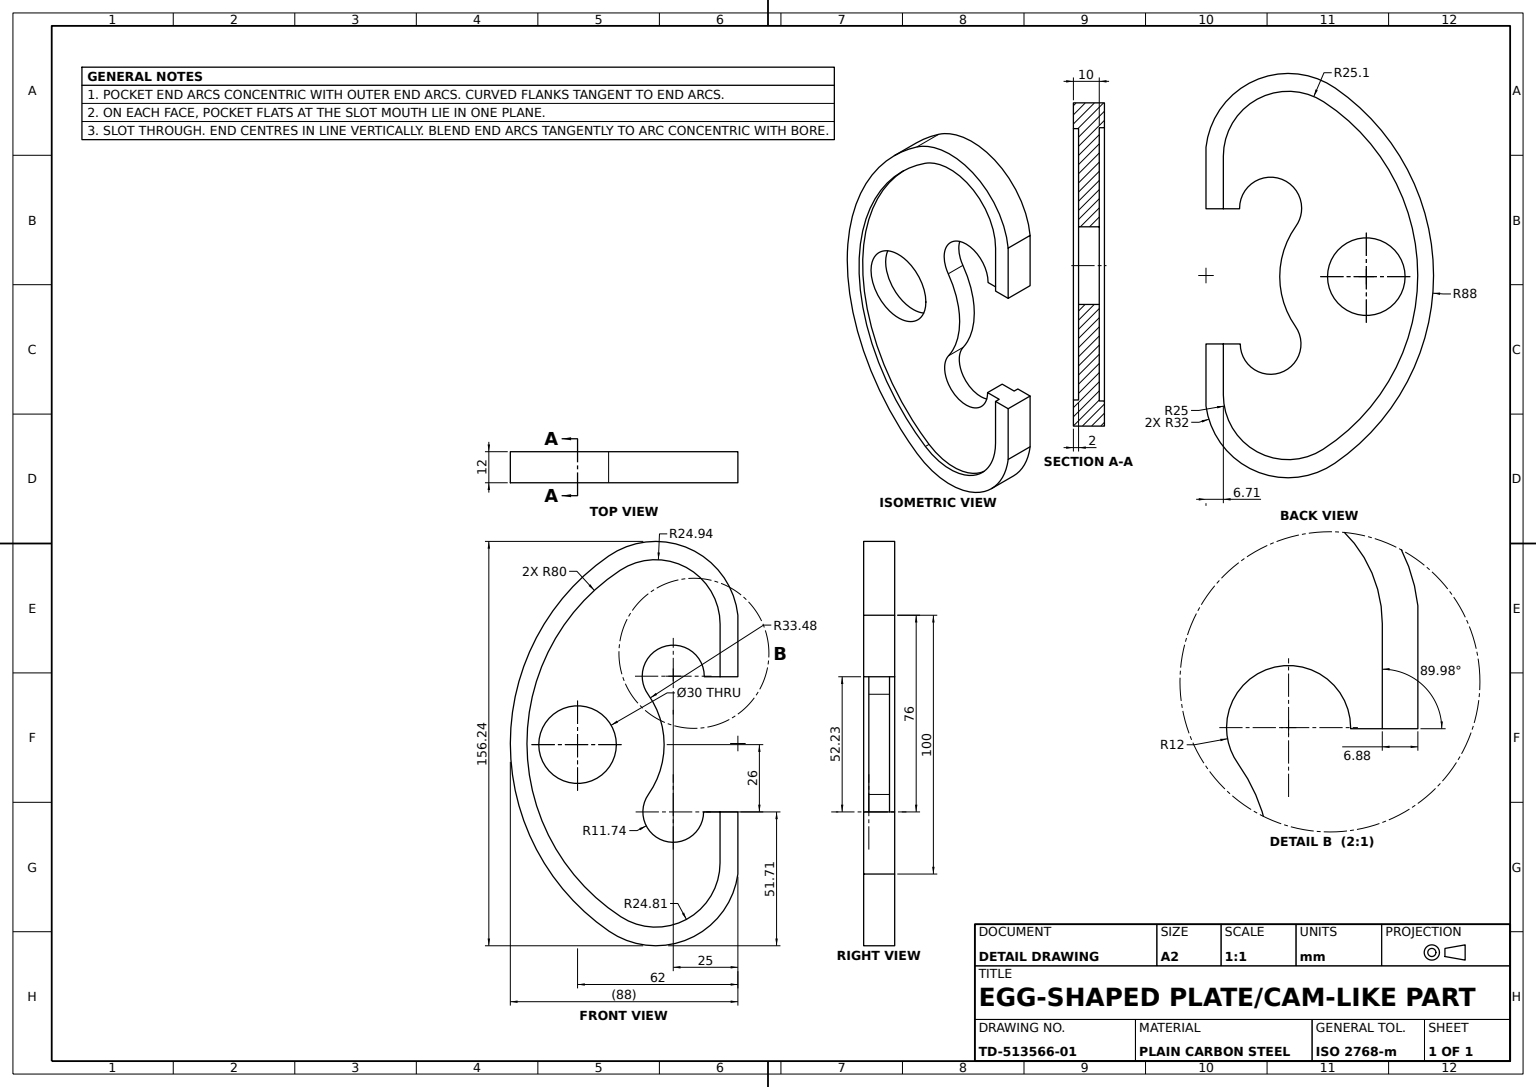
SolidWorks part; units mm, degrees
material "Plain Carbon Steel"
ref_plane "Front Plane" through (0, 0, 0) normal (0, 0, 1) x (1, 0, 0)
ref_plane "Top Plane" through (0, 0, 0) normal (0, 1, 0) x (1, 0, 0)
ref_plane "Right Plane" through (0, 0, 0) normal (1, 0, 0) x (0, 0, -1)
sketch "Plate Outline Sketch" plane through (0, 0, 0) normal (0, 0, 1) x (1, 0, 0)
  line L0 (0, 0) -> (0, -76)
  line L1 (0, 0) -> (0, 11.5583)
  line L2 (0, -76) -> (0, -88.4417)
  arc A0 (0, 11.5583) -> (-31.8112, 40.0874) centre (-31.8112, 8.0874) ccw
  arc A1 (-31.7117, -116.1559) -> (0, -88.4417) centre (-31.7117, -84.1559) ccw
  arc A2 (-49.989, 34.423) -> (-49.8327, -110.5307) centre (0, -38) ccw
  arc A3 (0, 11.5583) -> (-49.989, 34.423) centre (-31.8112, 8.0874) ccw
  arc A4 (-49.8327, -110.5307) -> (0, -88.4417) centre (-31.7117, -84.1559) ccw
  dimension "D1" = 88
  dimension "D2" = 32
  dimension "D3" = 32
  dimension "D4" = 100
  dimension "D5" = 76
  dimension "D6" = 22.089
extrude "Plate Body 12mm" add sketch "Plate Outline Sketch" along normal blind 12 contours A2 A4 A1 L2 L0 L1 A0 A3
sketch "Through Hole Sketch" plane through (0, 0, 12) normal (0, 0, 1) x (1, 0, 0)
  circle A0 centre (-62, -38.4417) radius 15
  dimension "D1" = 30
  dimension "D2" = 62
  dimension "D3" = 72.8648
extrude "Through Hole" cut sketch "Through Hole Sketch" against normal blind 12
sketch "Face Pocket A Sketch" plane through (0, 0, 12) normal (0, 0, 1) x (1, 0, 0)
  line L2 (-6.8735, 8.0803) -> (-6.8997, -84.163)
  arc A1 (-6.8735, 8.0803) -> (-45.5078, 28.9271) centre (-31.8112, 8.0874) ccw
  arc A2 (-45.2634, -104.9401) -> (-6.8997, -84.163) centre (-31.7117, -84.1559) ccw
  arc A3 (-45.5078, 28.9271) -> (-45.2634, -104.9401) centre (-1.5693, -37.9265) ccw
  dimension "D1" = 80
  dimension "D2" = 24.9377
  dimension "D3" = 24.812
  dimension "D4" = 80
extrude "Face Pocket A 2mm" cut sketch "Face Pocket A Sketch" against normal blind 2
sketch "Face Pocket B Sketch" plane through (0, 0, 0) normal (0, 0, -1) x (-1, 0, 0)
  line L0 (6.7117, 8.0874) -> (6.7117, -84.1559)
  arc A0 (45.4907, 29.1315) -> (6.7117, 8.0874) centre (31.8112, 8.0874) ccw
  arc A1 (6.7117, -84.1559) -> (45.2671, -105.1619) centre (31.7117, -84.1559) ccw
  arc A2 (45.4907, 29.1315) -> (45.2671, -105.1619) centre (1.8898, -37.9428) cw
  dimension "D1" = 80
  dimension "D2" = 25.0995
  dimension "D4" = 80
extrude "Face Pocket B 2mm" cut sketch "Face Pocket B Sketch" against normal blind 2
sketch "Slot Opening Sketch" plane through (0, 0, 10) normal (0, 0, 1) x (1, 0, 0)
  line L3 (-12.998, -12.2121) -> (-6.8793, -12.2121)
  line L5 (-6.8997, -84.163) -> (-6.8735, 8.0803) construction
  line L7 (-13.2586, -64.4417) -> (-6.8941, -64.4417)
  line L9 (-6.8941, -64.4417) -> (0, -64.4417)
  line L10 (0, 11.5583) -> (0, -88.4417) construction
  line L11 (0, -64.4417) -> (0, -12.2121)
  line L12 (0, -12.2121) -> (-6.8793, -12.2121)
  arc A0 (-34.6068, -57.6911) -> (-34.7596, -18.9767) centre (-62, -38.4417) ccw
  arc A2 (-12.998, -12.2121) -> (-34.7596, -18.9767) centre (-24.9961, -12.0001) ccw
  arc A3 (-34.6068, -57.6911) -> (-13.2586, -64.4417) centre (-25, -64.4417) ccw
  dimension "D1" = 33.4802
  dimension "D2" = 12
  dimension "D3" = 11.7414
  dimension "D4" = 10.7482
  dimension "D5" = 10.901
  dimension "D6" = 32.5098
extrude "Slot Opening Cut" cut sketch "Slot Opening Sketch" against normal blind 10
sketch "Rim Notch A Sketch" plane through (0, 0, 10) normal (0, 0, -1) x (-1, 0, 0)
  line L0 (0, -12.2121) -> (6.7117, -12.2121)
  line L1 (6.7117, -12.2121) -> (6.7117, -64.4417)
  line L2 (6.7117, -64.4417) -> (0, -64.4417)
  line L3 (0, -64.4417) -> (0, -12.2121)
extrude "Rim Notch A" cut sketch "Rim Notch A Sketch" against normal blind 10
sketch "Rim Notch B Sketch" plane through (-6.7117, 0, 0) normal (1, 0, 0) x (0, 0, -1)
  line L0 (-12, -12.2121) -> (-10, -12.2121)
  line L1 (-10, -12.2121) -> (-10, -64.4417)
  line L2 (-10, -64.4417) -> (-12, -64.4417)
  line L3 (-12, -64.4417) -> (-12, -12.2121)
extrude "Rim Notch B" cut sketch "Rim Notch B Sketch" against normal blind 10
